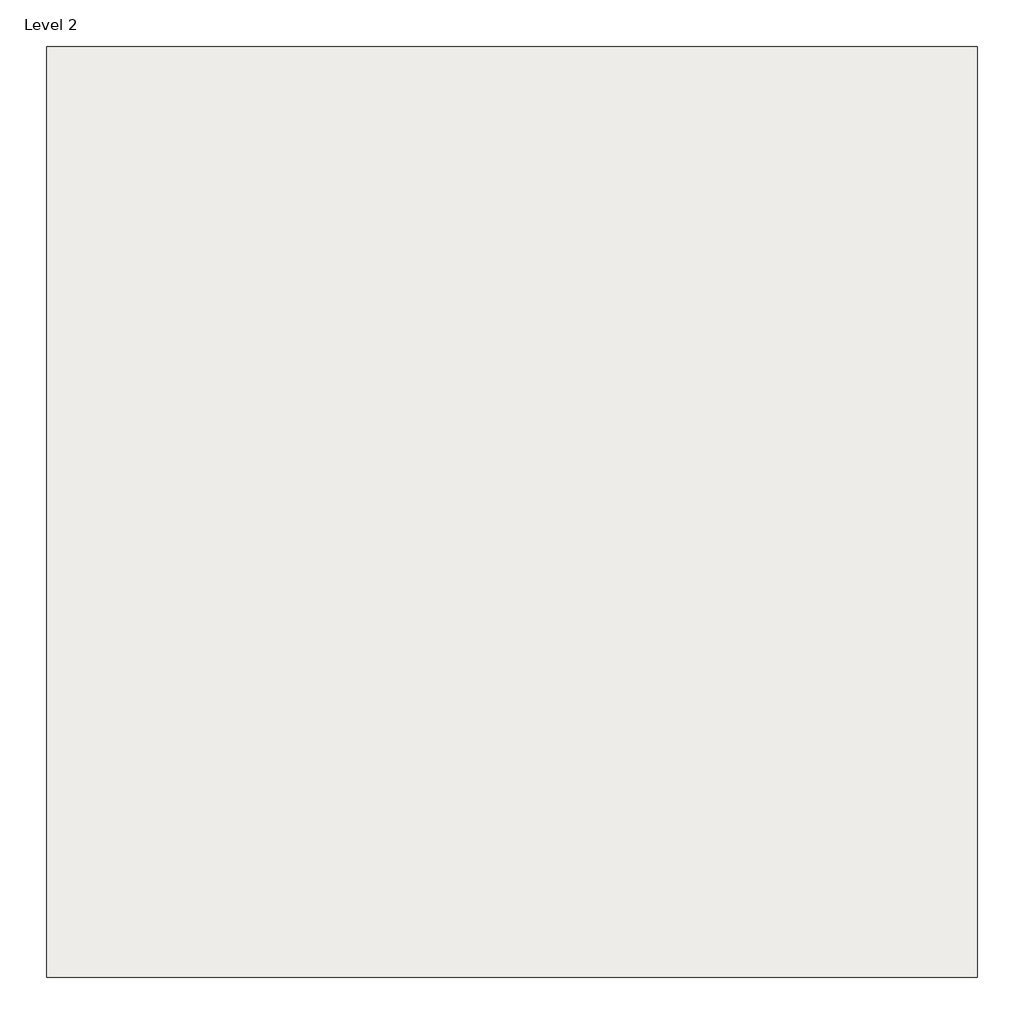
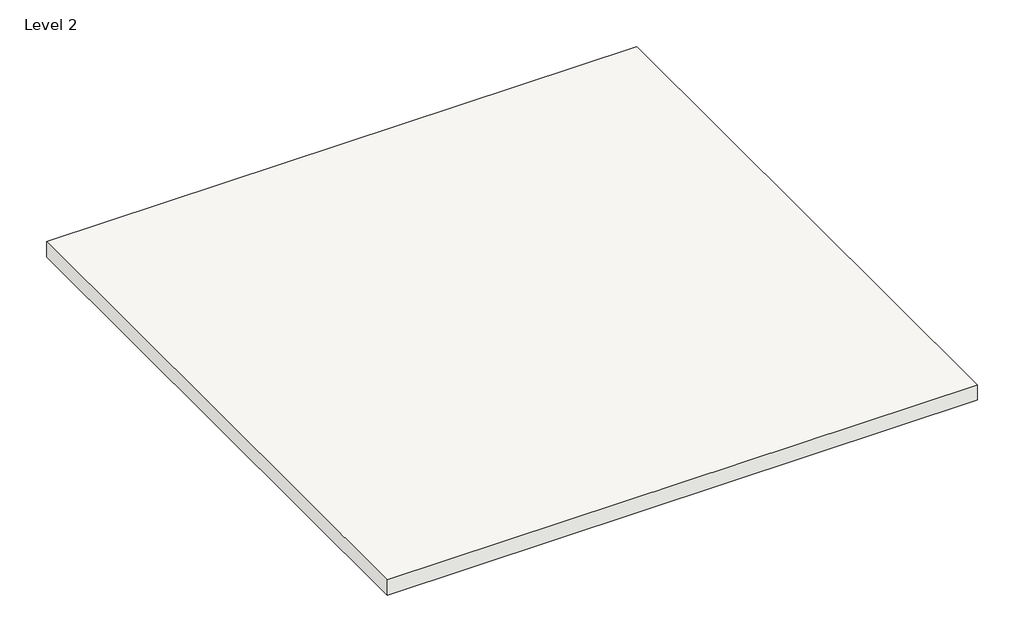
# One storey: 1 roof.
"""IFC4 building model written with IfcOpenShell, lengths in millimetres."""

from ifc_helpers import new_model, si_unit, frame, origin, place, context, project, spatial, polyline, outline, extrude, element, save

model = new_model("IFC4")

# Units and contexts
model_context = context("Model", 3, world=origin())
ifc_project = project(units=[si_unit("LENGTHUNIT", "METRE", prefix="MILLI")], contexts=[model_context])

# Site, building, storey
site = spatial("IfcSite", under=ifc_project)
building = spatial("IfcBuilding", under=site)
storey = spatial("IfcBuildingStorey", under=building, Name="Level 2", Elevation=3048.0)

# Roof
placement = place(None, origin())
element("IfcRoof", 1, ObjectType="Generic - 12\"", at=placement, inside=storey, context=model_context, shape_type="SweptSolid", body=[
    extrude(outline(polyline([(-17559.9067057, 13410.3187882), (-6383.9067057, 13410.3187882), (-6383.9067057, 2234.3187882), (-17559.9067057, 2234.3187882), (-17559.9067057, 13410.3187882)])), frame((0.0, 0.0, 3048.0), z_axis=(0.0, 0.0, 1.0), x_axis=(1.0, 0.0, 0.0)), (0.0, 0.0, 1.0), 304.8),
])

save(model, "model.ifc")

# Revit data of these elements
# Type "Generic - 12\""
#   Assembly Code = "B1020"
#   Layers, outside or top first: 1' - 0" "Brick, Soldier Course" (function 1)
# Element 1 (IfcRoof, "Generic - 12\"")
#   built-in parameter 1001705 = 11 (stored number, unit not read)
#   built-in parameter 1001710 = 33615
#   Phase Created = New Construction
#   Materials on its faces: "Brick, Soldier Course"
# Materials
#   "Brick, Soldier Course": class "Masonry", colour RGB 170 98 104, transparency 0, Description = "Common brick soldier coursed", Cost = 0
